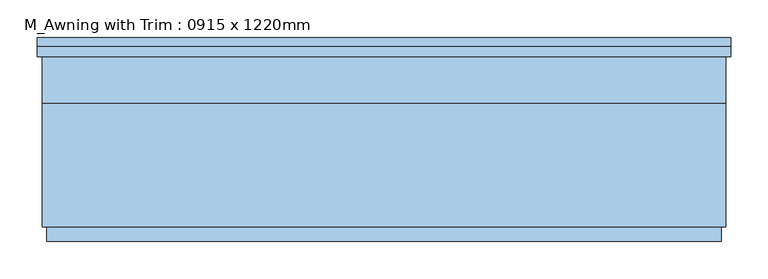
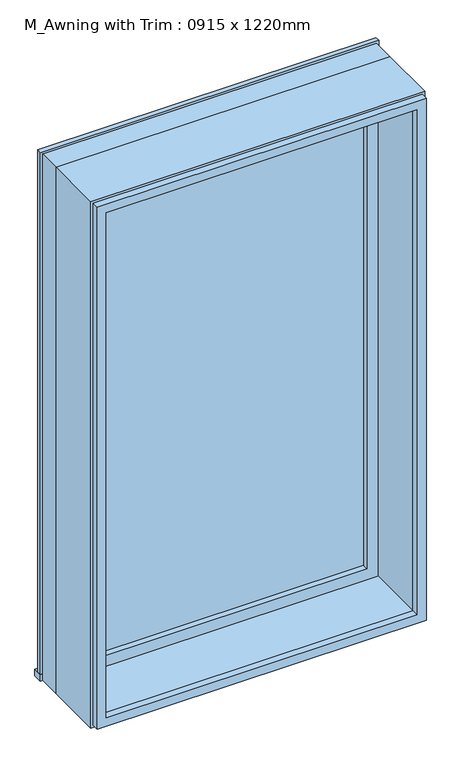
"""IFC4 building model written with IfcOpenShell, lengths in millimetres: window geometry, M_Awning with Trim : 0915 x 1220mm."""

from ifc_helpers import new_model, si_unit, frame, origin, place, context, project, spatial, polyline, outline, extrude, source, transform, mapped, element, save


def m_awning_with_trim_0915_x_1220mm_6739fb62(model_context):
    return source(origin(), model_context, "Body", "SweptSolid", [
        extrude(outline(polyline([(-463.85, 140.0), (463.85, 140.0), (463.85, 114.3), (-463.85, 114.3), (-463.85, 140.0)])), frame((0.0, 0.0, 915.0), z_axis=(0.0, 0.0, 1.0), x_axis=(1.0, 0.0, 0.0)), (0.0, 0.0, 1.0), 19.05),
        extrude(outline(polyline([(2419.95, -438.45), (2419.95, 438.45), (934.05, 438.45), (934.05, 463.85), (2445.35, 463.85), (2445.35, -463.85), (934.05, -463.85), (934.05, -438.45), (2419.95, -438.45)])), frame((0.0, 114.3, 0.0), z_axis=(0.0, 1.0, 0.0), x_axis=(0.0, 0.0, 1.0)), (0.0, 0.0, 1.0), 13.0),
        extrude(outline(polyline([(2432.65, 451.15), (2432.65, -451.15), (921.35, -451.15), (921.35, 451.15), (2432.65, 451.15)]), holes=[polyline([(2407.25, 425.75), (946.75, 425.75), (946.75, -425.75), (2407.25, -425.75), (2407.25, 425.75)])]), frame((0.0, -133.3, 0.0), z_axis=(0.0, 1.0, 0.0), x_axis=(0.0, 0.0, 1.0)), (0.0, 0.0, 1.0), 19.0),
        extrude(outline(polyline([(394.0, 66.725), (-394.0, 66.725), (-394.0, 79.425), (394.0, 79.425), (394.0, 66.725)])), frame((0.0, 0.0, 978.5), z_axis=(0.0, 0.0, 1.0), x_axis=(1.0, 0.0, 0.0)), (0.0, 0.0, 1.0), 1397.0),
        extrude(outline(polyline([(2419.95, -438.45), (934.05, -438.45), (934.05, 438.45), (2419.95, 438.45), (2419.95, -438.45)]), holes=[polyline([(2375.5, -394.0), (2375.5, 394.0), (978.5, 394.0), (978.5, -394.0), (2375.5, -394.0)])]), frame((0.0, 50.85, 0.0), z_axis=(0.0, 1.0, 0.0), x_axis=(0.0, 0.0, 1.0)), (0.0, 0.0, 1.0), 44.45),
        extrude(outline(polyline([(2439.0, -457.5), (915.0, -457.5), (915.0, 457.5), (2439.0, 457.5), (2439.0, -457.5)]), holes=[polyline([(2407.25, -425.75), (2407.25, 425.75), (946.75, 425.75), (946.75, -425.75), (2407.25, -425.75)])]), frame((0.0, -114.3, 0.0), z_axis=(0.0, 1.0, 0.0), x_axis=(0.0, 0.0, 1.0)), (0.0, 0.0, 1.0), 165.15),
        extrude(outline(polyline([(2439.0, 457.5), (2439.0, -457.5), (915.0, -457.5), (915.0, 457.5), (2439.0, 457.5)]), holes=[polyline([(2419.95, 438.45), (934.05, 438.45), (934.05, -438.45), (2419.95, -438.45), (2419.95, 438.45)])]), frame((0.0, 50.85, 0.0), z_axis=(0.0, 1.0, 0.0), x_axis=(0.0, 0.0, 1.0)), (0.0, 0.0, 1.0), 63.45),
    ])


if __name__ == "__main__":
    model = new_model("IFC4")
    model_context = context("Model", 3, world=origin())
    ifc_project = project(units=[si_unit("LENGTHUNIT", "METRE", prefix="MILLI")], contexts=[model_context])
    site = spatial("IfcSite", under=ifc_project)
    building = spatial("IfcBuilding", under=site)
    placement = place(None, origin())
    m_awning_with_trim_0915_x_1220mm_shape = m_awning_with_trim_0915_x_1220mm_6739fb62(model_context)
    element("IfcWindow", 1, ObjectType="M_Awning with Trim : 0915 x 1220mm", at=placement, inside=building, context=model_context, shape_type="MappedRepresentation", body=[
        mapped(m_awning_with_trim_0915_x_1220mm_shape, transform((0.0, 0.0, 0.0), x_axis=(1.0, 0.0, 0.0), y_axis=(0.0, 1.0, 0.0), z_axis=(0.0, 0.0, 1.0))),
    ])
    save(model, "model.ifc")

# Revit data of these elements
# Type "M_Awning with Trim : 0915 x 1220mm"
#   Type Mark = "13"
#   Construction Type Id = "GSP4R"
#   Analytic Construction = "1/8 in Pilkington single glazing"
#   Visual Light Transmittance = 0.9
#   Solar Heat Gain Coefficient = 0.78
#   Heat Transfer Coefficient (U) = 0.6496 BTU/(h·ft²·°F)
#   Height = 5' - 0"
#   Default Sill Height = 3' - 0.02362"
#   Trim Projection - Ext. = 0' - 0.51181"
#   Trim Projection - Int. = 0' - 0.74803"
#   Trim Width - Exterior = 0' - 1"
#   Trim Width - Interior = 0' - 1"
#   Width = 3' - 0.02362"
#   Window Inset = 0' - 0.74803"
#   Define Thermal Properties by = 1
#   Glass Pane Material = Glass
#   Sash = Sash
#   Trim Exterior Material = Trim
#   Trim Interior Material = Trim
#   Wall Closure = (empty or 0)
# Element 1 (IfcWindow, "M_Awning with Trim : 0915 x 1220mm")
#   Materials on its faces: "Trim", "Sash", "Glass"
# Materials
#   "Glass": class "Glass", colour RGB 0 128 192, transparency 0.75, Description = "Soda Lime Glass", Cost = 0
#   "Sash": class "Wood", colour RGB 224 178 126, transparency 0
#   "Trim": class "Wood", colour RGB 224 178 126, transparency 0
